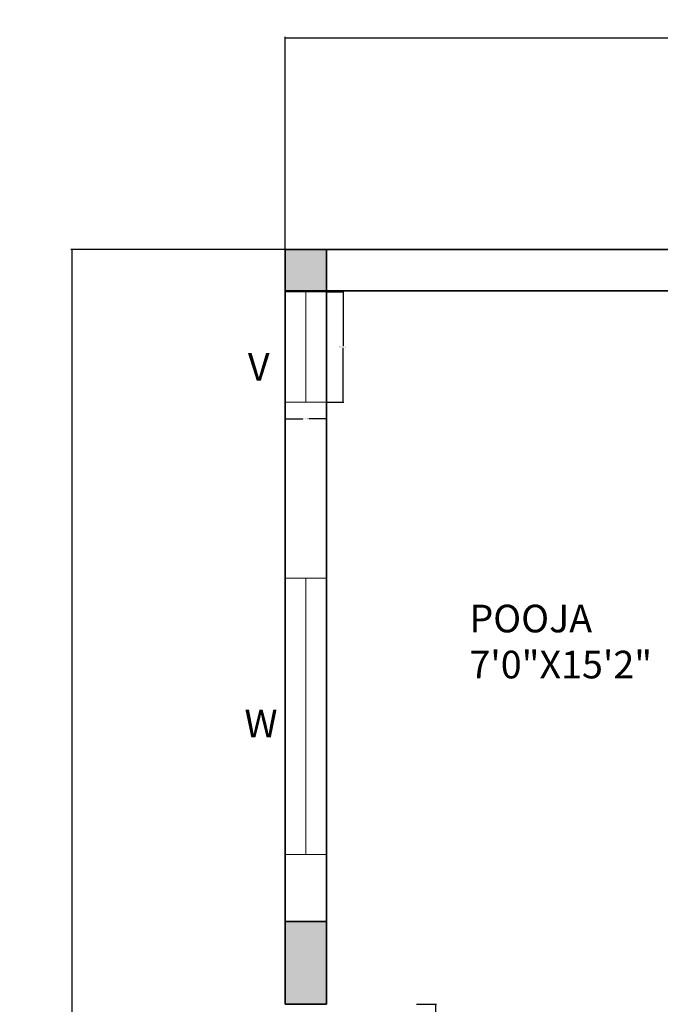
# Model space of a CAD drawing. Units: inches. Extents: x -36302355 to 648, y -221479757 to 75.
# Tile 29 of 37: x 87 to 227, y -139 to 75. Entities that reach past the tile are written whole.
import ezdxf

# ---------------------------------------------------------------- set-up
doc = ezdxf.new("R2010")
doc.units = ezdxf.units.IN
doc.header["$MEASUREMENT"] = 0
for name, color, linetype, lineweight in [('A-ANNO-DIMS', 2, 'Continuous', 18), ('A-ANNO-IDEN', 7, 'Continuous', 18), ('A-AREA-IDEN', 7, 'Continuous', 18), ('A-COLS', 7, 'Continuous', 35), ('A-COLS-PATT', 242, 'Continuous', 13), ('A-GLAZ', 142, 'Continuous', 18), ('A-WALL', 7, 'Continuous', 35)]:
    doc.layers.add(name, color=color, linetype=linetype, lineweight=lineweight)
doc.styles.get("Standard").update_dxf_attribs({"font": 'arial.ttf'})
doc.dimstyles.get("Standard").update_dxf_attribs({"dimtxt": 0.18, "dimasz": 0.18, "dimexe": 0.18, "dimexo": 0.0625, "dimgap": 0.09, "dimtad": 0, "dimtih": 1, "dimtoh": 1, "dimdec": 0, "dimzin": 0, "dimdsep": 46, "dimlunit": 3, "dimtxsty": 'Standard', "dimcen": 0.09, "dimadec": 0, "dimazin": 0, "dimtfac": 1, "dimtdec": 0, "dimtofl": 0, "dimtmove": 0, "dimatfit": 3, "dimfxl": 1, "dimtolj": 1, "dimtzin": 0, "dimarcsym": 0})

# ---------------------------------------------------------------- blocks, each defined once
blk = doc.blocks.new('*D4')
at = {"layer": 'A-ANNO-DIMS', "color": 0, "lineweight": -2, "transparency": 16777216}
for p, q in [((145.2, 25.04), (145.2, 71.11)), ((145.38, 70.93), (364.8, 70.93)), ((605.02, 70.93), (385.59, 70.93)), ((605.2, 25.04), (605.2, 71.11))]:
    blk.add_line(p, q, dxfattribs=at)
at = {"layer": 'A-ANNO-DIMS', "color": 0, "transparency": 16777216}
for points in [[(145.38, 70.96), (145.38, 70.9), (145.2, 70.93)], [(605.02, 70.96), (605.02, 70.9), (605.2, 70.93)]]:
    blk.add_solid(points, dxfattribs=at)
at = {"layer": 'Defpoints', "color": 0, "transparency": 16777216}
for p in [(605.2, 70.93), (145.2, 24.98), (605.2, 24.98)]:
    blk.add_point(p, dxfattribs=at)
at = {"layer": 'A-ANNO-DIMS', "color": 0, "transparency": 16777216, "insert": (375.2, 70.93), "char_height": 6, "attachment_point": 5}
blk.add_mtext('\\A1;38\'-4"', dxfattribs=at)
blk = doc.blocks.new('*D7')
at = {"layer": 'A-ANNO-DIMS', "color": 0, "lineweight": -2, "transparency": 16777216}
for p, q in [((145.13, 24.98), (98.63, 24.98)), ((98.81, 24.8), (98.81, -274.37)), ((98.81, -579.84), (98.81, -280.67)), ((145.13, -580.02), (98.63, -580.02))]:
    blk.add_line(p, q, dxfattribs=at)
at = {"layer": 'A-ANNO-DIMS', "color": 0, "transparency": 16777216}
for points in [[(98.78, 24.8), (98.84, 24.8), (98.81, 24.98)], [(98.78, -579.84), (98.84, -579.84), (98.81, -580.02)]]:
    blk.add_solid(points, dxfattribs=at)
at = {"layer": 'Defpoints', "color": 0, "transparency": 16777216}
for p in [(98.81, 24.98), (145.2, 24.98), (145.2, -580.02)]:
    blk.add_point(p, dxfattribs=at)
at = {"layer": 'A-ANNO-DIMS', "color": 0, "transparency": 16777216, "insert": (98.81, -277.52), "char_height": 6, "attachment_point": 5}
blk.add_mtext('\\A1;50\'-5"', dxfattribs=at)
blk = doc.blocks.new('WIN-60')
for p, q in [((60, 9), (0, 9)), ((0, 9), (0, 0)), ((60, 0), (60, 9)), ((0, 4.5), (60, 4.5)), ((0, 0), (60, 0))]:
    blk.add_line(p, q)
blk = doc.blocks.new('VENT-24')
for p, q in [((0, 0), (0, 24)), ((0, 24), (9, 24)), ((4.5, 24), (4.5, 0)), ((9, 24), (9, 0)), ((9, 0), (0, 0))]:
    blk.add_line(p, q)
blk = doc.blocks.new('*D25')
at = {"layer": 'A-ANNO-DIMS', "color": 0, "lineweight": -2, "transparency": 16777216}
for p, q in [((173.76, -139.02), (178.08, -139.02)), ((177.9, -139.2), (177.9, -152.84)), ((177.9, -166.84), (177.9, -153.2)), ((173.76, -167.02), (178.08, -167.02))]:
    blk.add_line(p, q, dxfattribs=at)
at = {"layer": 'A-ANNO-DIMS', "color": 0, "transparency": 16777216}
for points in [[(177.87, -139.2), (177.93, -139.2), (177.9, -139.02)], [(177.87, -166.84), (177.93, -166.84), (177.9, -167.02)]]:
    blk.add_solid(points, dxfattribs=at)
at = {"layer": 'Defpoints', "color": 0, "transparency": 16777216}
for p in [(173.7, -139.02), (177.9, -139.02), (173.7, -167.02)]:
    blk.add_point(p, dxfattribs=at)
at = {"layer": 'A-ANNO-DIMS', "color": 0, "transparency": 16777216, "insert": (177.9, -153.02), "char_height": 0.18, "attachment_point": 5}
blk.add_mtext('\\A1;SWING DOOR 2\'-4" TYP.', dxfattribs=at)
blk = doc.blocks.new('*D49')
at = {"layer": 'A-ANNO-DIMS', "color": 0, "lineweight": -2, "transparency": 16777216}
for p, q in [((154.26, 15.78), (157.98, 15.78)), ((157.8, 15.6), (157.8, 3.96)), ((157.8, -8.04), (157.8, 3.6)), ((154.26, -8.22), (157.98, -8.22))]:
    blk.add_line(p, q, dxfattribs=at)
at = {"layer": 'A-ANNO-DIMS', "color": 0, "transparency": 16777216}
for points in [[(157.77, 15.6), (157.83, 15.6), (157.8, 15.78)], [(157.77, -8.04), (157.83, -8.04), (157.8, -8.22)]]:
    blk.add_solid(points, dxfattribs=at)
at = {"layer": 'Defpoints', "color": 0, "transparency": 16777216}
for p in [(154.2, 15.78), (157.8, 15.78), (154.2, -8.22)]:
    blk.add_point(p, dxfattribs=at)
at = {"layer": 'A-ANNO-DIMS', "color": 0, "transparency": 16777216, "insert": (157.8, 3.78), "char_height": 0.18, "attachment_point": 5}
blk.add_mtext('\\A1;VENT 2\'-0" TYP.', dxfattribs=at)
blk = doc.blocks.new('*D50')
at = {"layer": 'A-ANNO-DIMS', "color": 0, "lineweight": -2, "transparency": 16777216}
for p, q in [((145.2, -8.29), (145.2, -12)), ((154.2, -8.29), (154.2, -12)), ((145.38, -11.82), (149.06, -11.82)), ((154.02, -11.82), (150.34, -11.82))]:
    blk.add_line(p, q, dxfattribs=at)
at = {"layer": 'A-ANNO-DIMS', "color": 0, "transparency": 16777216}
for points in [[(145.38, -11.79), (145.38, -11.85), (145.2, -11.82)], [(154.02, -11.79), (154.02, -11.85), (154.2, -11.82)]]:
    blk.add_solid(points, dxfattribs=at)
at = {"layer": 'Defpoints', "color": 0, "transparency": 16777216}
for p in [(145.2, -8.22), (154.2, -8.22), (154.2, -11.82)]:
    blk.add_point(p, dxfattribs=at)
at = {"layer": 'A-ANNO-DIMS', "color": 0, "transparency": 16777216, "insert": (149.7, -11.82), "char_height": 0.18, "attachment_point": 5}
blk.add_mtext('\\A1;0\'-9" TYP.', dxfattribs=at)

msp = doc.modelspace()

# ---------------------------------------------------------------- hatches: boundary and pattern name
at = {"layer": 'A-COLS-PATT'}
h = msp.add_hatch(color=256, dxfattribs=at)
h.dxf.hatch_style = 1
h.paths.add_polyline_path([(145.2, 24.98), (145.2, 15.98), (154.2, 15.98), (154.2, 24.98)])
h.paths.add_polyline_path([(247.2, 15.98), (247.2, 24.98), (238.2, 24.98), (238.2, 15.98)])
h.paths.add_polyline_path([(387.64, 15.98), (395.7, 15.98), (395.7, 24.98), (387.64, 24.98)])
h.paths.add_polyline_path([(451.26, 24.98), (443.7, 24.98), (443.7, 15.98), (451.26, 15.98)])
h.paths.add_polyline_path([(596.2, 15.98), (605.2, 15.98), (605.2, 24.98), (596.2, 24.98)])
h.paths.add_polyline_path([(238.2, -122.02), (238.2, -131.02), (247.2, -131.02), (247.2, -122.02)])
h.paths.add_polyline_path([(395.7, -122.02), (387.46, -122.02), (387.46, -131.02), (395.7, -131.02)])
h.paths.add_polyline_path([(448.2, -131.02), (453.73, -131.02), (453.73, -122.02), (443.7, -122.02), (443.7, -131.02)])
h.paths.add_polyline_path([(596.2, -131.02), (605.2, -131.02), (605.2, -122.02), (596.2, -122.02)])
h.paths.add_polyline_path([(145.2, -176.97), (154.2, -176.97), (154.2, -167.02), (145.2, -167.02)])
h.paths.add_polyline_path([(314.2, -176.97), (323.2, -176.97), (323.2, -167.02), (314.2, -167.02)])
h.paths.add_polyline_path([(154.2, -314.02), (154.2, -309.52), (145.2, -309.52), (145.2, -314.02)])
h.paths.add_polyline_path([(314.2, -309.52), (314.2, -318.52), (323.2, -318.52), (323.2, -309.52)])
h.paths.add_polyline_path([(448.2, -277.02), (443.7, -277.02), (443.7, -286.02), (448.2, -286.02)])
h.paths.add_polyline_path([(283.2, -370.02), (274.2, -370.02), (274.2, -379.02), (283.2, -379.02), (283.2, -374.52)])
h.paths.add_polyline_path([(154.2, -370.02), (145.2, -370.02), (145.2, -379.02), (154.2, -379.02)])
h.paths.add_polyline_path([(443.2, -374.52), (443.2, -379.02), (452.2, -379.02), (452.2, -374.52)])
h.paths.add_polyline_path([(145.2, -580.02), (154.2, -580.02), (154.2, -571.02), (145.2, -571.02)])
h.paths.add_polyline_path([(274.2, -571.02), (274.2, -580.02), (283.2, -580.02), (283.2, -571.02)])
h.paths.add_polyline_path([(443.2, -580.02), (452.2, -580.02), (452.2, -571.02), (443.2, -571.02)])
h = msp.add_hatch(color=256, dxfattribs=at)
h.dxf.hatch_style = 1
h.paths.add_polyline_path([(154.2, -121.04), (145.2, -121.04), (145.2, -139.02), (149.7, -139.02), (154.2, -139.02)])

# ---------------------------------------------------------------- linework, layer by layer
at = {"layer": 'A-COLS'}
for p, q in [((154.2, -121.04), (145.2, -121.04)), ((149.7, -139.02), (145.2, -139.02)), ((149.7, -139.02), (154.2, -139.02))]:
    msp.add_line(p, q, dxfattribs=at)
at = {"layer": 'A-WALL'}
for p, q in [((145.2, 24.98), (145.2, -139.02)), ((145.2, 24.98), (605.2, 24.98)), ((154.2, 24.98), (154.2, -139.02)), ((145.2, 15.98), (605.2, 15.98))]:
    msp.add_line(p, q, dxfattribs=at)

# ---------------------------------------------------------------- block references
at = {"layer": 'A-GLAZ'}
msp.add_blockref('VENT-24', (145.2, -8.22), dxfattribs=at)
at = {"layer": 'A-GLAZ', "extrusion": (0, 0, -1), "zscale": -1, "rotation": 90}
msp.add_blockref('WIN-60', (-145.2, -106.45), dxfattribs=at)

# ---------------------------------------------------------------- texts
at = {"layer": 'A-ANNO-IDEN', "char_height": 6, "attachment_point": 1}
for s, insert in [('V', (137.11, 2.44)), ('W', (136.36, -75.03))]:
    msp.add_mtext(s, dxfattribs=dict(at, insert=insert))
at = {"layer": 'A-AREA-IDEN', "insert": (185.25, -52.22), "char_height": 6, "attachment_point": 1}
msp.add_mtext('POOJA\\P7\'0"X15\'2"', dxfattribs=at)

# ---------------------------------------------------------------- dimensions: what is measured, and where the dimension line sits
at = {"layer": 'A-ANNO-DIMS'}
dim = msp.add_linear_dim(base=(605.2, 70.93), p1=(145.2, 24.98), p2=(605.2, 24.98), dimstyle='Standard', override={"dimtxt": 6, "dimclrd": 0, "dimclre": 0, "dimclrt": 0}, dxfattribs=at)
dim.commit()
dim.dimension.update_dxf_attribs({"geometry": '*D4', "text_midpoint": (375.2, 70.93)})
dim = msp.add_linear_dim(base=(98.81, 24.98), p1=(145.2, -580.02), p2=(145.2, 24.98), angle=90, dimstyle='Standard', override={"dimtxt": 6, "dimclrd": 0, "dimclre": 0, "dimclrt": 0}, dxfattribs=at)
dim.commit()
dim.dimension.update_dxf_attribs({"geometry": '*D7', "text_midpoint": (98.81, -277.52)})
for base, p1, p2, text, picture, middle in [((157.8, 15.78), (154.2, -8.22), (154.2, 15.78), 'VENT <> TYP.', '*D49', (157.8, 3.78)), ((177.9, -139.02), (173.7, -167.02), (173.7, -139.02), 'SWING DOOR <> TYP.', '*D25', (177.9, -153.02))]:
    dim = msp.add_linear_dim(base=base, p1=p1, p2=p2, angle=90, text=text, dimstyle='Standard', override={"dimdec": 1, "dimlfac": 1, "dimrnd": 0, "dimzin": 1, "dimdsep": 46, "dimlunit": 4, "dimfrac": 2}, dxfattribs=at)
    dim.commit()
    dim.dimension.update_dxf_attribs({"geometry": picture, "text_midpoint": middle})
dim = msp.add_linear_dim(base=(154.2, -11.82), p1=(145.2, -8.22), p2=(154.2, -8.22), text='<> TYP.', dimstyle='Standard', override={"dimdec": 1, "dimlfac": 1, "dimrnd": 0, "dimzin": 1, "dimdsep": 46, "dimlunit": 4, "dimfrac": 2}, dxfattribs=at)
dim.commit()
dim.dimension.update_dxf_attribs({"geometry": '*D50', "text_midpoint": (149.7, -11.82)})

doc.saveas('drawing.dxf')
